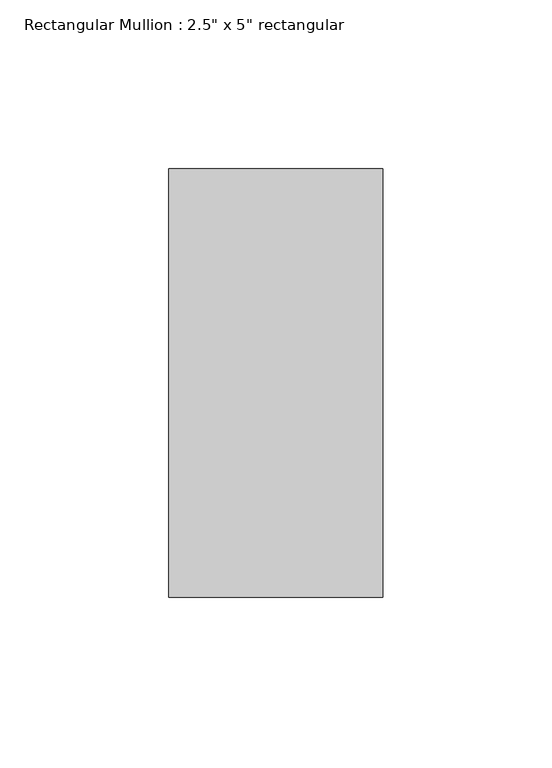
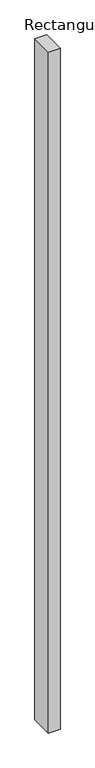
"""IFC4 building model written with IfcOpenShell, lengths in millimetres: member geometry."""

from ifc_helpers import new_model, si_unit, frame, origin, place, context, project, spatial, polyline, outline, extrude, source, transform, mapped, element, save


def member_63be31b3(model_context):
    return source(origin(), model_context, "Body", "SweptSolid", [
        extrude(outline(polyline([(0.0, 63.5), (0.0, -63.5), (-63.5, -63.5), (-63.5, 63.5), (0.0, 63.5)])), frame((0.0, 0.0, -3911.6), z_axis=(0.0, 0.0, 1.0), x_axis=(1.0, 0.0, 0.0)), (0.0, 0.0, 1.0), 3911.6),
    ])


if __name__ == "__main__":
    model = new_model("IFC4")
    model_context = context("Model", 3, world=origin())
    ifc_project = project(units=[si_unit("LENGTHUNIT", "METRE", prefix="MILLI")], contexts=[model_context])
    site = spatial("IfcSite", under=ifc_project)
    building = spatial("IfcBuilding", under=site)
    placement = place(None, origin())
    member_shape = member_63be31b3(model_context)
    element("IfcMember", 1, ObjectType="Rectangular Mullion : 2.5\" x 5\" rectangular", at=placement, inside=building, context=model_context, shape_type="MappedRepresentation", body=[
        mapped(member_shape, transform((0.0, 0.0, 0.0), x_axis=(1.0, 0.0, 0.0), y_axis=(0.0, 1.0, 0.0), z_axis=(0.0, 0.0, 1.0))),
    ])
    save(model, "model.ifc")

# Revit data of these elements
# Type "Rectangular Mullion : 2.5\" x 5\" rectangular"
#   built-in parameter 1007304 = 0.416667 (stored number, unit not read)
#   built-in parameter 1007301 = 0.104167 (stored number, unit not read)
#   built-in parameter 1007300 = 0.104167 (stored number, unit not read)
